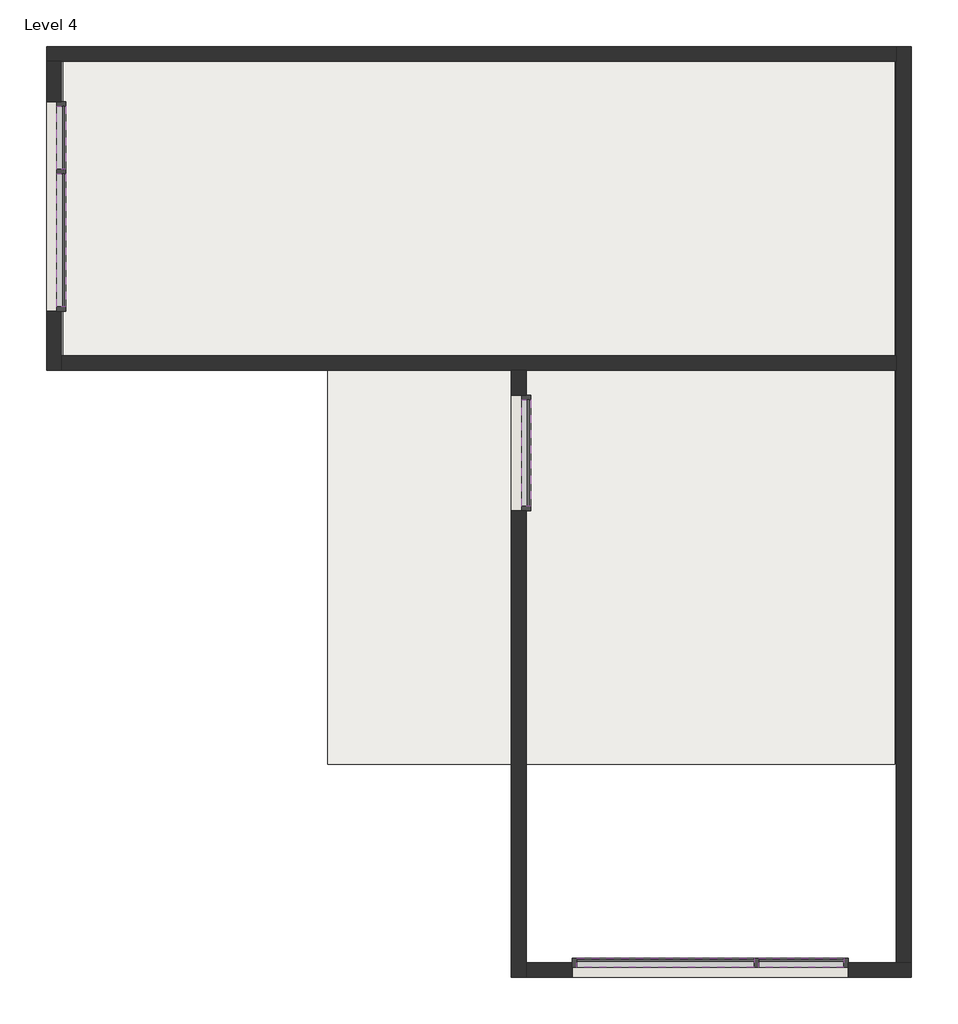
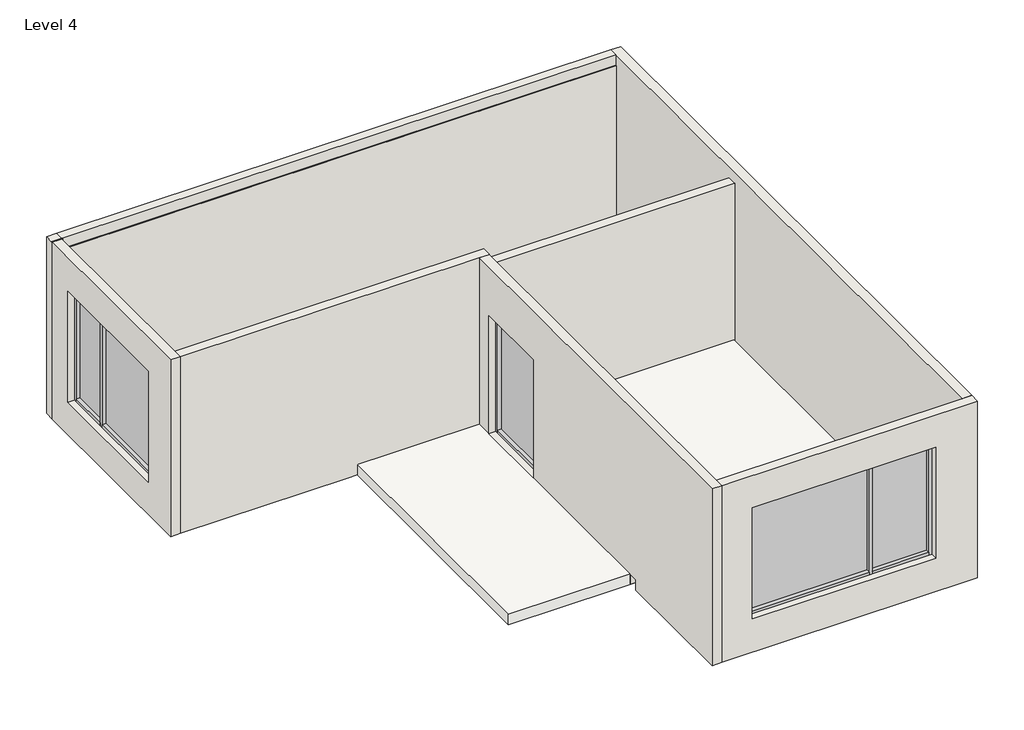
# One storey: 18 members, 6 walls, 5 plates, 1 roof.
"""IFC4 building model written with IfcOpenShell, lengths in millimetres."""

from ifc_helpers import new_model, si_unit, frame, origin, place, context, project, spatial, polyline, outline, extrude, faceted_brep, transform, mapped, element, save
from components import member_f0fea5a5, member_ee409385, member_f6bf76ec, member_8dcffc12, member_91d29dfe, member_3e16bac7, member_75351bdb, member_024c663a, system_panel_glazed_21a81833, system_panel_glazed_0b5a89bb, system_panel_glazed_010dc334, system_panel_glazed_9c94e0d4, system_panel_glazed_98faf640

model = new_model("IFC4")

# Units and contexts
model_context = context("Model", 3, world=origin())
ifc_project = project(units=[si_unit("LENGTHUNIT", "METRE", prefix="MILLI")], contexts=[model_context])

# Site, building, storey
site = spatial("IfcSite", under=ifc_project)
building = spatial("IfcBuilding", under=site)
storey = spatial("IfcBuildingStorey", under=building, Name="Level 4", Elevation=10972.8)

# Members
placement = place(None, origin())
member_shape = member_f0fea5a5(model_context)
element("IfcMember", 1, ObjectType="Rectangular Mullion : 2.5\" x 5\" rectangular", at=placement, inside=storey, context=model_context, shape_type="MappedRepresentation", body=[
    mapped(member_shape, transform((-6507.5589554, -4832.7372168, 11709.103192), x_axis=(1.0, 0.0, 0.0), y_axis=(0.0, -1.0, 0.0), z_axis=(0.0, 0.0, -1.0))),
])
element("IfcMember", 2, ObjectType="Rectangular Mullion : 2.5\" x 5\" rectangular", at=placement, inside=storey, context=model_context, shape_type="MappedRepresentation", body=[
    mapped(member_shape, transform((-16104.8624512, 6092.2679989, 11676.0763898), x_axis=(0.0, -1.0, 0.0), y_axis=(-1.0, 0.0, 0.0), z_axis=(0.0, 0.0, -1.0))),
])
member_2_shape = member_ee409385(model_context)
element("IfcMember", 3, ObjectType="Rectangular Mullion : 2.5\" x 5\" rectangular", at=placement, inside=storey, context=model_context, shape_type="MappedRepresentation", body=[
    mapped(member_2_shape, transform((-5236.9376844, -4832.7372168, 11709.103192), x_axis=(1.0, 0.0, 0.0), y_axis=(0.0, -1.0, 0.0), z_axis=(0.0, 0.0, -1.0))),
])
element("IfcMember", 4, ObjectType="Rectangular Mullion : 2.5\" x 5\" rectangular", at=placement, inside=storey, context=model_context, shape_type="MappedRepresentation", body=[
    mapped(member_2_shape, transform((-16104.8624512, 4161.8679989, 11676.0763898), x_axis=(0.0, -1.0, 0.0), y_axis=(-1.0, 0.0, 0.0), z_axis=(0.0, 0.0, -1.0))),
])
element("IfcMember", 5, ObjectType="Rectangular Mullion : 2.5\" x 5\" rectangular", at=placement, inside=storey, context=model_context, shape_type="MappedRepresentation", body=[
    mapped(member_2_shape, transform((-9048.8014975, -4832.7372168, 14147.503192), x_axis=(-1.0, 0.0, 0.0), y_axis=(0.0, -1.0, 0.0), z_axis=(0.0, 0.0, 1.0))),
])
element("IfcMember", 6, ObjectType="Rectangular Mullion : 2.5\" x 5\" rectangular", at=placement, inside=storey, context=model_context, shape_type="MappedRepresentation", body=[
    mapped(member_2_shape, transform((-16104.8624512, 7057.4679989, 14114.4763898), x_axis=(0.0, 1.0, 0.0), y_axis=(-1.0, 0.0, 0.0), z_axis=(0.0, 0.0, 1.0))),
])
member_3_shape = member_f6bf76ec(model_context)
element("IfcMember", 7, ObjectType="Rectangular Mullion : 2.5\" x 5\" rectangular", at=placement, inside=storey, context=model_context, shape_type="MappedRepresentation", body=[
    mapped(member_3_shape, transform((-5300.4376844, -4832.7372168, 14147.503192), x_axis=(0.0, 0.0, 1.0), y_axis=(0.0, -1.0, 0.0), z_axis=(1.0, 0.0, 0.0))),
])
element("IfcMember", 8, ObjectType="Rectangular Mullion : 2.5\" x 5\" rectangular", at=placement, inside=storey, context=model_context, shape_type="MappedRepresentation", body=[
    mapped(member_3_shape, transform((-6475.8089554, -4832.7372168, 11709.103192), x_axis=(0.0, 0.0, -1.0), y_axis=(0.0, -1.0, 0.0), z_axis=(-1.0, 0.0, 0.0))),
])
member_4_shape = member_8dcffc12(model_context)
element("IfcMember", 9, ObjectType="Rectangular Mullion : 2.5\" x 5\" rectangular", at=placement, inside=storey, context=model_context, shape_type="MappedRepresentation", body=[
    mapped(member_4_shape, transform((-6539.3089554, -4832.7372168, 14147.503192), x_axis=(0.0, 0.0, 1.0), y_axis=(0.0, -1.0, 0.0), z_axis=(1.0, 0.0, 0.0))),
])
element("IfcMember", 10, ObjectType="Rectangular Mullion : 2.5\" x 5\" rectangular", at=placement, inside=storey, context=model_context, shape_type="MappedRepresentation", body=[
    mapped(member_4_shape, transform((-8985.3014975, -4832.7372168, 11709.103192), x_axis=(0.0, 0.0, -1.0), y_axis=(0.0, -1.0, 0.0), z_axis=(-1.0, 0.0, 0.0))),
])
member_5_shape = member_91d29dfe(model_context)
element("IfcMember", 11, ObjectType="Rectangular Mullion : 2.5\" x 5\" rectangular", at=placement, inside=storey, context=model_context, shape_type="MappedRepresentation", body=[
    mapped(member_5_shape, transform((-9686.8372956, 1467.908754, 13789.128654), x_axis=(0.0, 0.0, 1.0), y_axis=(-1.0, 0.0, 0.0), z_axis=(0.0, -1.0, 0.0))),
])
element("IfcMember", 12, ObjectType="Rectangular Mullion : 2.5\" x 5\" rectangular", at=placement, inside=storey, context=model_context, shape_type="MappedRepresentation", body=[
    mapped(member_5_shape, transform((-9686.8372956, 2936.6903521, 11201.4), x_axis=(0.0, 0.0, -1.0), y_axis=(-1.0, 0.0, 0.0), z_axis=(0.0, 1.0, 0.0))),
])
member_6_shape = member_3e16bac7(model_context)
element("IfcMember", 13, ObjectType="Rectangular Mullion : 2.5\" x 5\" rectangular", at=placement, inside=storey, context=model_context, shape_type="MappedRepresentation", body=[
    mapped(member_6_shape, transform((-9686.8372956, 1404.408754, 11201.4), x_axis=(0.0, -1.0, 0.0), y_axis=(-1.0, 0.0, 0.0), z_axis=(0.0, 0.0, -1.0))),
])
element("IfcMember", 14, ObjectType="Rectangular Mullion : 2.5\" x 5\" rectangular", at=placement, inside=storey, context=model_context, shape_type="MappedRepresentation", body=[
    mapped(member_6_shape, transform((-9686.8372956, 3000.1903521, 13789.128654), x_axis=(0.0, 1.0, 0.0), y_axis=(-1.0, 0.0, 0.0), z_axis=(0.0, 0.0, 1.0))),
])
member_7_shape = member_75351bdb(model_context)
element("IfcMember", 15, ObjectType="Rectangular Mullion : 2.5\" x 5\" rectangular", at=placement, inside=storey, context=model_context, shape_type="MappedRepresentation", body=[
    mapped(member_7_shape, transform((-16104.8624512, 6060.5179989, 11676.0763898), x_axis=(0.0, 0.0, -1.0), y_axis=(-1.0, 0.0, 0.0), z_axis=(0.0, 1.0, 0.0))),
])
member_8_shape = member_024c663a(model_context)
element("IfcMember", 16, ObjectType="Rectangular Mullion : 2.5\" x 5\" rectangular", at=placement, inside=storey, context=model_context, shape_type="MappedRepresentation", body=[
    mapped(member_8_shape, transform((-16104.8624512, 6993.9679989, 11676.0763898), x_axis=(0.0, 0.0, -1.0), y_axis=(-1.0, 0.0, 0.0), z_axis=(0.0, 1.0, 0.0))),
])
element("IfcMember", 17, ObjectType="Rectangular Mullion : 2.5\" x 5\" rectangular", at=placement, inside=storey, context=model_context, shape_type="MappedRepresentation", body=[
    mapped(member_8_shape, transform((-16104.8624512, 6124.0179989, 14114.4763898), x_axis=(0.0, 0.0, 1.0), y_axis=(-1.0, 0.0, 0.0), z_axis=(0.0, -1.0, 0.0))),
])
element("IfcMember", 18, ObjectType="Rectangular Mullion : 2.5\" x 5\" rectangular", at=placement, inside=storey, context=model_context, shape_type="MappedRepresentation", body=[
    mapped(member_7_shape, transform((-16104.8624512, 4225.3679989, 14114.4763898), x_axis=(0.0, 0.0, 1.0), y_axis=(-1.0, 0.0, 0.0), z_axis=(0.0, -1.0, 0.0))),
])

# Plates
system_panel_glazed_shape = system_panel_glazed_21a81833(model_context)
element("IfcPlate", 19, ObjectType="System Panel : Glazed", at=placement, inside=storey, context=model_context, shape_type="MappedRepresentation", body=[
    mapped(system_panel_glazed_shape, transform((-5888.1233199, -4832.7372168, 11772.603192), x_axis=(1.0, 0.0, 0.0), y_axis=(0.0, 1.0, 0.0), z_axis=(0.0, 0.0, 1.0))),
])
system_panel_glazed_2_shape = system_panel_glazed_0b5a89bb(model_context)
element("IfcPlate", 20, ObjectType="System Panel : Glazed", at=placement, inside=storey, context=model_context, shape_type="MappedRepresentation", body=[
    mapped(system_panel_glazed_2_shape, transform((-7762.3052265, -4832.7372168, 11772.603192), x_axis=(1.0, 0.0, 0.0), y_axis=(0.0, 1.0, 0.0), z_axis=(0.0, 0.0, 1.0))),
])
system_panel_glazed_3_shape = system_panel_glazed_010dc334(model_context)
element("IfcPlate", 21, ObjectType="System Panel : Glazed", at=placement, inside=storey, context=model_context, shape_type="MappedRepresentation", body=[
    mapped(system_panel_glazed_3_shape, transform((-9686.8372956, 2202.2995531, 11264.9), x_axis=(0.0, -1.0, 0.0), y_axis=(1.0, 0.0, 0.0), z_axis=(0.0, 0.0, 1.0))),
])
system_panel_glazed_4_shape = system_panel_glazed_9c94e0d4(model_context)
element("IfcPlate", 22, ObjectType="System Panel : Glazed", at=placement, inside=storey, context=model_context, shape_type="MappedRepresentation", body=[
    mapped(system_panel_glazed_4_shape, transform((-16104.8624512, 6558.9929989, 11739.5763898), x_axis=(0.0, -1.0, 0.0), y_axis=(1.0, 0.0, 0.0), z_axis=(0.0, 0.0, 1.0))),
])
system_panel_glazed_5_shape = system_panel_glazed_98faf640(model_context)
element("IfcPlate", 23, ObjectType="System Panel : Glazed", at=placement, inside=storey, context=model_context, shape_type="MappedRepresentation", body=[
    mapped(system_panel_glazed_5_shape, transform((-16104.8624512, 5142.9429989, 11739.5763898), x_axis=(0.0, -1.0, 0.0), y_axis=(1.0, 0.0, 0.0), z_axis=(0.0, 0.0, 1.0))),
])

# Roof
element("IfcRoof", 24, ObjectType="Generic - 9\"", at=placement, inside=storey, context=model_context, shape_type="SweptSolid", body=[
    extrude(outline(polyline([(-12633.2372956, 7613.2627832), (-5876.8372956, 7613.2627832), (-4598.6624512, 7613.2627832), (-4598.6624512, -2089.5372168), (-5876.8372956, -2089.5372168), (-12423.6872956, -2089.5372168), (-12423.6872956, 3549.2627832), (-16079.4624512, 3549.2627832), (-16079.4624512, 7613.2627832), (-12633.2372956, 7613.2627832)])), frame((0.0, 0.0, 10972.8), z_axis=(0.0, 0.0, 1.0), x_axis=(1.0, 0.0, 0.0)), (0.0, 0.0, 1.0), 228.6),
])

# Walls
element("IfcWall", 25, ObjectType="Generic - 8\"", at=placement, inside=storey, context=model_context, shape_type="Brep", body=[
    faceted_brep([(-16308.0624512, 7613.2627832, 10972.8), (-16104.8624512, 7613.2627832, 10972.8), (-4573.2624512, 7613.2627832, 10972.8), (-4573.2624512, 7613.2627832, 14630.4), (-16092.1624512, 7613.2627832, 14630.4), (-16092.1624512, 7613.2627832, 14859.0), (-16104.8624512, 7613.2627832, 14859.0), (-16308.0624512, 7613.2627832, 14859.0), (-16308.0624512, 7816.4627832, 10972.8), (-16308.0624512, 7816.4627832, 14859.0), (-16092.1624512, 7816.4627832, 14859.0), (-4573.2624512, 7816.4627832, 14859.0), (-4573.2624512, 7816.4627832, 10972.8), (-16308.0624512, 7638.6627832, 14859.0), (-4573.2624512, 7638.6627832, 14859.0), (-4573.2624512, 7638.6627832, 14630.4), (-16092.1624512, 7638.6627832, 14859.0), (-16092.1624512, 7638.6627832, 14630.4)], [[[0, 1, 2, 3, 4, 5, 6, 7]], [[8, 9, 10, 11, 12]], [[2, 1, 0, 8, 12]], [[0, 7, 13, 9, 8]], [[3, 2, 12, 11, 14, 15]], [[14, 16, 17, 15]], [[7, 6, 5, 16, 13]], [[16, 5, 4, 17]], [[14, 11, 10, 16]], [[10, 9, 13, 16]], [[4, 3, 15, 17]]]),
])
element("IfcWall", 26, ObjectType="Generic - 8\"", at=placement, inside=storey, context=model_context, shape_type="Brep", body=[
    faceted_brep([(-16104.8624512, 3346.0627832, 10972.8), (-16104.8624512, 3549.2627832, 10972.8), (-16104.8624512, 7613.2627832, 10972.8), (-16104.8624512, 7613.2627832, 14859.0), (-16104.8624512, 3549.2627832, 14859.0), (-16104.8624512, 3346.0627832, 14859.0), (-16104.8624512, 4161.8679989, 14114.4763898), (-16104.8624512, 7057.4679989, 14114.4763898), (-16104.8624512, 7057.4679989, 11676.0763898), (-16104.8624512, 4161.8679989, 11676.0763898), (-16308.0624512, 3346.0627832, 10972.8), (-16308.0624512, 3346.0627832, 14859.0), (-16308.0624512, 7613.2627832, 14859.0), (-16308.0624512, 7613.2627832, 10972.8), (-16308.0624512, 4161.8679989, 14114.4763898), (-16308.0624512, 4161.8679989, 11676.0763898), (-16308.0624512, 7057.4679989, 11676.0763898), (-16308.0624512, 7057.4679989, 14114.4763898)], [[[0, 1, 2, 3, 4, 5], [6, 7, 8, 9]], [[10, 11, 12, 13], [14, 15, 16, 17]], [[0, 5, 11, 10]], [[3, 2, 13, 12]], [[2, 1, 0, 10, 13]], [[5, 4, 3, 12, 11]], [[7, 6, 14, 17]], [[8, 7, 17, 16]], [[9, 8, 16, 15]], [[6, 9, 15, 14]]]),
])
element("IfcWall", 27, ObjectType="Generic - 8\"", at=placement, inside=storey, context=model_context, shape_type="Brep", body=[
    faceted_brep([(-4573.2624512, 3549.2627832, 10972.8), (-16104.8624512, 3549.2627832, 10972.8), (-16104.8624512, 3549.2627832, 14859.0), (-9680.4872956, 3549.2627832, 14859.0), (-9680.4872956, 3549.2627832, 14630.4), (-4573.2624512, 3549.2627832, 14630.4), (-4573.2624512, 3346.0627832, 10972.8), (-4573.2624512, 3346.0627832, 14630.4), (-9680.4872956, 3346.0627832, 14630.4), (-9680.4872956, 3346.0627832, 14859.0), (-9686.8372956, 3346.0627832, 14859.0), (-9890.0372956, 3346.0627832, 14859.0), (-16104.8624512, 3346.0627832, 14859.0), (-16104.8624512, 3346.0627832, 10972.8), (-12633.2372956, 3346.0627832, 10972.8), (-12430.0372956, 3346.0627832, 10972.8), (-9890.0372956, 3346.0627832, 10972.8), (-9686.8372956, 3346.0627832, 10972.8)], [[[0, 1, 2, 3, 4, 5]], [[6, 7, 8, 9, 10, 11, 12, 13, 14, 15, 16, 17]], [[1, 0, 6, 17, 16, 15, 14, 13]], [[0, 5, 7, 6]], [[2, 1, 13, 12]], [[3, 2, 12, 11, 10, 9]], [[3, 9, 8, 4]], [[5, 4, 8, 7]]]),
])
element("IfcWall", 28, ObjectType="Generic - 8\"", at=placement, inside=storey, context=model_context, shape_type="Brep", body=[
    faceted_brep([(-4573.2624512, 7816.4627832, 10972.8), (-4573.2624512, 7613.2627832, 10972.8), (-4573.2624512, 3549.2627832, 10972.8), (-4573.2624512, 3346.0627832, 10972.8), (-4573.2624512, -4832.7372168, 10972.8), (-4573.2624512, -4832.7372168, 14859.0), (-4573.2624512, 7638.6627832, 14859.0), (-4573.2624512, 7816.4627832, 14859.0), (-4370.0624512, 7816.4627832, 10972.8), (-4370.0624512, 7816.4627832, 14859.0), (-4370.0624512, -4832.7372168, 14859.0), (-4370.0624512, -4832.7372168, 10972.8)], [[[0, 1, 2, 3, 4, 5, 6, 7]], [[8, 9, 10, 11]], [[4, 3, 2, 1, 0, 8, 11]], [[7, 6, 5, 10, 9]], [[0, 7, 9, 8]], [[5, 4, 11, 10]]]),
])
element("IfcWall", 29, ObjectType="Generic - 8\"", at=placement, inside=storey, context=model_context, shape_type="Brep", body=[
    faceted_brep([(-9890.0372956, 3346.0627832, 10972.8), (-9890.0372956, -2089.5372168, 10972.8), (-9890.0372956, -2089.5372168, 11201.4), (-9890.0372956, -2292.7372168, 11201.4), (-9890.0372956, -2292.7372168, 10972.8), (-9890.0372956, -5035.9372168, 10972.8), (-9890.0372956, -5035.9372168, 14859.0), (-9890.0372956, 3346.0627832, 14859.0), (-9890.0372956, 1404.408754, 13789.128654), (-9890.0372956, 1404.408754, 11201.4), (-9890.0372956, 3000.1903521, 11201.4), (-9890.0372956, 3000.1903521, 13789.128654), (-9686.8372956, 3346.0627832, 10972.8), (-9686.8372956, 3346.0627832, 14859.0), (-9686.8372956, -4832.7372168, 14859.0), (-9686.8372956, -5035.9372168, 14859.0), (-9686.8372956, -5035.9372168, 10972.8), (-9686.8372956, -4832.7372168, 10972.8), (-9686.8372956, -2292.7372168, 10972.8), (-9686.8372956, -2292.7372168, 11201.4), (-9686.8372956, -2089.5372168, 11201.4), (-9686.8372956, -2089.5372168, 10972.8), (-9686.8372956, 1404.408754, 13789.128654), (-9686.8372956, 3000.1903521, 13789.128654), (-9686.8372956, 3000.1903521, 11201.4), (-9686.8372956, 1404.408754, 11201.4), (-9788.4372956, -2292.7372168, 10972.8)], [[[0, 1, 2, 3, 4, 5, 6, 7], [8, 9, 10, 11]], [[12, 13, 14, 15, 16, 17, 18, 19, 20, 21], [22, 23, 24, 25]], [[0, 7, 13, 12]], [[6, 5, 16, 15]], [[1, 0, 12, 21]], [[7, 6, 15, 14, 13]], [[2, 1, 21, 20]], [[3, 2, 20, 19]], [[5, 4, 26, 18, 17, 16]], [[4, 3, 19, 18, 26]], [[9, 8, 22, 25]], [[10, 9, 25, 24]], [[11, 10, 24, 23]], [[8, 11, 23, 22]]]),
])
element("IfcWall", 30, ObjectType="Generic - 8\"", at=placement, inside=storey, context=model_context, shape_type="Brep", body=[
    faceted_brep([(-9686.8372956, -5035.9372168, 10972.8), (-4370.0624512, -5035.9372168, 10972.8), (-4370.0624512, -5035.9372168, 14859.0), (-9686.8372956, -5035.9372168, 14859.0), (-5236.9376844, -5035.9372168, 14147.503192), (-5236.9376844, -5035.9372168, 11709.103192), (-9048.8014975, -5035.9372168, 11709.103192), (-9048.8014975, -5035.9372168, 14147.503192), (-9686.8372956, -4832.7372168, 10972.8), (-9686.8372956, -4832.7372168, 14859.0), (-4573.2624512, -4832.7372168, 14859.0), (-4370.0624512, -4832.7372168, 14859.0), (-4370.0624512, -4832.7372168, 10972.8), (-4573.2624512, -4832.7372168, 10972.8), (-5236.9376844, -4832.7372168, 14147.503192), (-9048.8014975, -4832.7372168, 14147.503192), (-9048.8014975, -4832.7372168, 11709.103192), (-5236.9376844, -4832.7372168, 11709.103192)], [[[0, 1, 2, 3], [4, 5, 6, 7]], [[8, 9, 10, 11, 12, 13], [14, 15, 16, 17]], [[0, 3, 9, 8]], [[2, 1, 12, 11]], [[1, 0, 8, 13, 12]], [[3, 2, 11, 10, 9]], [[5, 4, 14, 17]], [[6, 5, 17, 16]], [[7, 6, 16, 15]], [[4, 7, 15, 14]]]),
])

save(model, "model.ifc")

# Revit data of these elements
# Type "Rectangular Mullion : 2.5\" x 5\" rectangular"
#   built-in parameter 1007304 = 0.416667 (stored number, unit not read)
#   built-in parameter 1007301 = 0.104167 (stored number, unit not read)
#   built-in parameter 1007300 = 0.104167 (stored number, unit not read)
# Type "System Panel : Glazed"
#   Construction Type Id = "GSP4R"
#   Analytic Construction = "1/8 in Pilkington single glazing"
#   Visual Light Transmittance = 0.9
#   Solar Heat Gain Coefficient = 0.86
#   Heat Transfer Coefficient (U) = 1.18115 BTU/(h·ft²·°F)
# Type "Generic - 9\""
#   Assembly Code = "B1020"
#   Layers, outside or top first: 0' - 9" no material (function 1)
# Type "Generic - 8\""
#   Assembly Code = "B2010"
#   Layers, outside or top first: 0' - 8" no material (function 1)
# Elements 1, 2, 3, 4, 5, 6, 7, 8, 9, 10, 11, 12, 13, 14, 15, 16, 17, 18 (IfcMember, "Rectangular Mullion : 2.5\" x 5\" rectangular")
#   Phase Created = New Construction
#   Materials on its faces: "Aluminum"
# Elements 19, 20, 21, 22, 23 (IfcPlate, "System Panel : Glazed")
#   Phase Created = New Construction
#   Materials on its faces: "Glass"
# Element 24 (IfcRoof, "Generic - 9\"")
#   built-in parameter 1001705 = 36.75 (stored number, unit not read)
#   built-in parameter 1001710 = 33615
#   Phase Created = New Construction
#   Materials on its faces: "Default Roof", "Cherry"
# Elements 25, 26, 27, 28, 29, 30 (IfcWall, "Generic - 8\"")
#   Top Offset = 0' - 0"
#   Base Offset = 0' - 0"
#   Unconnected Height = 12' - 9"
#   wall height = 12' - 9"
#   Phase Created = New Construction
#   Base Constraint = Level 4
#   Materials on its faces: "Default Wall", "Cherry"
# Materials
#   "Aluminum": class "Metal", colour RGB 247 247 247, transparency 0, Description = "Aluminum 6061", Cost = 0
#   "Glass": class "Glass", colour RGB 0 128 192, transparency 0.75, Description = "Soda Lime Glass", Cost = 0
#   "Default Roof": colour RGB 88 101 114, transparency 0
#   "Cherry": class "Wood", colour RGB 226 177 128, transparency 0, Description = "Prunus Serotina", Cost = 0
#   "Default Wall": colour RGB 128 128 128, transparency 0
